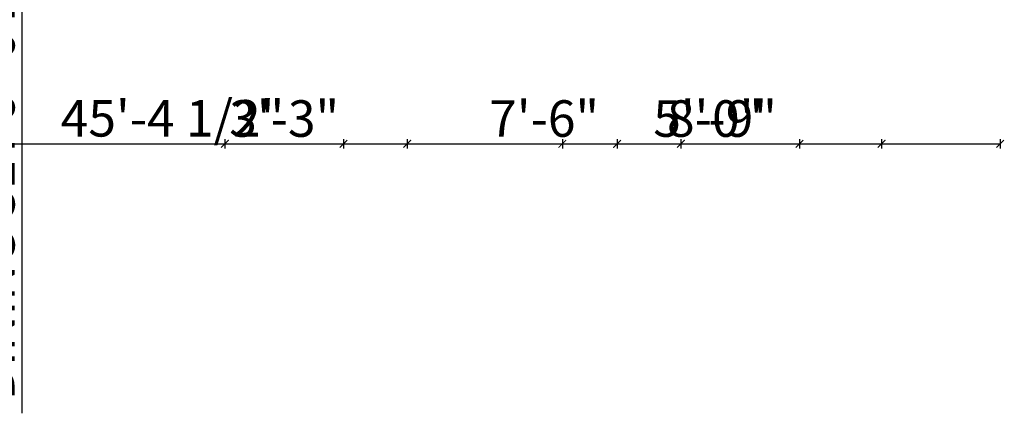
# Model space of a CAD drawing. Units: inches. Extents: x 375 to 1122, y 27 to 1069.
# Tile 6 of 155: x 667 to 990, y 27 to 157. Entities that reach past the tile are written whole.
import ezdxf

# ---------------------------------------------------------------- set-up
doc = ezdxf.new("R2010")
doc.units = ezdxf.units.IN
doc.layers.add('A-ANNO-DIMS', color=2, linetype='Continuous', lineweight=18)
doc.styles.get("Standard").update_dxf_attribs({"font": 'arial.ttf'})
doc.dimstyles.new('ISO-25', dxfattribs={"dimtxt": 12, "dimasz": 2.5, "dimexe": 1.5, "dimexo": 1.5, "dimtad": 1, "dimdec": 1, "dimlunit": 3, "dimtxsty": 'Standard', "dimblk": 'ARCHTICK', "dimcen": 2.5, "dimadec": 0, "dimazin": 0, "dimtfac": 1, "dimtdec": 1, "dimtmove": 0, "dimatfit": 3, "dimfxl": 1.5, "dimfxlon": 1, "dimarcsym": 0})

# ---------------------------------------------------------------- blocks, each defined once
blk = doc.blocks.new('_ArchTick')
at = {"color": 0, "linetype": 'ByBlock', "const_width": 0.15}
blk.add_lwpolyline([(-0.5, -0.5), (0.5, 0.5)], dxfattribs=at)
blk = doc.blocks.new('*D59')
at = {"layer": 'A-ANNO-DIMS', "color": 0, "lineweight": -2, "transparency": 16777216}
for p, q in [((668.72, 346.85), (665.72, 346.85)), ((667.22, 346.85), (667.22, 232.35)), ((668.72, 232.35), (665.72, 232.35)), ((667.22, 232.35), (667.22, 27.5))]:
    blk.add_line(p, q, dxfattribs=at)
at = {"layer": 'Defpoints', "color": 0, "transparency": 16777216}
for p in [(684.39, 346.85), (667.22, 232.35), (684.39, 232.35)]:
    blk.add_point(p, dxfattribs=at)
at = {"layer": 'A-ANNO-DIMS', "color": 0, "lineweight": -2, "transparency": 16777216, "xscale": 2.5, "yscale": 2.5, "zscale": 2.5}
for p, rotation in [((667.22, 346.85), 90), ((667.22, 232.35), 270)]:
    blk.add_blockref('_ArchTick', p, dxfattribs=dict(at, rotation=rotation))
at = {"layer": 'A-ANNO-DIMS', "color": 0, "transparency": 16777216, "insert": (660.39, 128.67), "char_height": 12, "attachment_point": 5, "rotation": 90}
blk.add_mtext('DINING SET 9\'-6 1/2" TYP.', dxfattribs=at)
blk = doc.blocks.new('*D81')
at = {"layer": 'A-ANNO-DIMS', "color": 0, "lineweight": -2, "transparency": 16777216}
for p, q in [((444.51, 117.53), (444.51, 114.53)), ((989.01, 117.53), (989.01, 114.53)), ((444.51, 116.03), (989.01, 116.03))]:
    blk.add_line(p, q, dxfattribs=at)
at = {"layer": 'Defpoints', "color": 0, "transparency": 16777216}
for p in [(444.51, 187.53), (989.01, 187.53), (989.01, 116.03)]:
    blk.add_point(p, dxfattribs=at)
at = {"layer": 'A-ANNO-DIMS', "color": 0, "lineweight": -2, "transparency": 16777216, "xscale": 2.5, "yscale": 2.5, "zscale": 2.5, "rotation": 180}
blk.add_blockref('_ArchTick', (444.51, 116.03), dxfattribs=at)
at = {"layer": 'A-ANNO-DIMS', "color": 0, "lineweight": -2, "transparency": 16777216, "xscale": 2.5, "yscale": 2.5, "zscale": 2.5}
blk.add_blockref('_ArchTick', (989.01, 116.03), dxfattribs=at)
at = {"layer": 'A-ANNO-DIMS', "color": 0, "transparency": 16777216, "insert": (716.76, 122.86), "char_height": 12, "attachment_point": 5}
blk.add_mtext('45\'-4 1/2"', dxfattribs=at)
blk = doc.blocks.new('*D84')
at = {"layer": 'A-ANNO-DIMS', "color": 0, "lineweight": -2, "transparency": 16777216}
for p, q in [((845.01, 117.53), (845.01, 114.53)), ((950.01, 117.53), (950.01, 114.53)), ((845.01, 116.03), (950.01, 116.03))]:
    blk.add_line(p, q, dxfattribs=at)
at = {"layer": 'Defpoints', "color": 0, "transparency": 16777216}
for p in [(845.01, 814.53), (950.01, 814.53), (950.01, 116.03)]:
    blk.add_point(p, dxfattribs=at)
at = {"layer": 'A-ANNO-DIMS', "color": 0, "lineweight": -2, "transparency": 16777216, "xscale": 2.5, "yscale": 2.5, "zscale": 2.5, "rotation": 180}
blk.add_blockref('_ArchTick', (845.01, 116.03), dxfattribs=at)
at = {"layer": 'A-ANNO-DIMS', "color": 0, "lineweight": -2, "transparency": 16777216, "xscale": 2.5, "yscale": 2.5, "zscale": 2.5}
blk.add_blockref('_ArchTick', (950.01, 116.03), dxfattribs=at)
at = {"layer": 'A-ANNO-DIMS', "color": 0, "transparency": 16777216, "insert": (897.51, 122.78), "char_height": 12, "attachment_point": 5}
blk.add_mtext('8\'-9"', dxfattribs=at)
blk = doc.blocks.new('*D87')
at = {"layer": 'A-ANNO-DIMS', "color": 0, "lineweight": -2, "transparency": 16777216}
for p, q in [((794.01, 117.53), (794.01, 114.53)), ((884.01, 117.53), (884.01, 114.53)), ((794.01, 116.03), (884.01, 116.03))]:
    blk.add_line(p, q, dxfattribs=at)
at = {"layer": 'Defpoints', "color": 0, "transparency": 16777216}
for p in [(794.01, 583.53), (884.01, 583.53), (884.01, 116.03)]:
    blk.add_point(p, dxfattribs=at)
at = {"layer": 'A-ANNO-DIMS', "color": 0, "lineweight": -2, "transparency": 16777216, "xscale": 2.5, "yscale": 2.5, "zscale": 2.5, "rotation": 180}
blk.add_blockref('_ArchTick', (794.01, 116.03), dxfattribs=at)
at = {"layer": 'A-ANNO-DIMS', "color": 0, "lineweight": -2, "transparency": 16777216, "xscale": 2.5, "yscale": 2.5, "zscale": 2.5}
blk.add_blockref('_ArchTick', (884.01, 116.03), dxfattribs=at)
at = {"layer": 'A-ANNO-DIMS', "color": 0, "transparency": 16777216, "insert": (839.01, 122.78), "char_height": 12, "attachment_point": 5}
blk.add_mtext('7\'-6"', dxfattribs=at)
blk = doc.blocks.new('*D89')
at = {"layer": 'A-ANNO-DIMS', "color": 0, "lineweight": -2, "transparency": 16777216}
for p, q in [((863.01, 117.53), (863.01, 114.53)), ((923.01, 117.53), (923.01, 114.53)), ((863.01, 116.03), (923.01, 116.03))]:
    blk.add_line(p, q, dxfattribs=at)
at = {"layer": 'Defpoints', "color": 0, "transparency": 16777216}
for p in [(863.01, 574.53), (923.01, 574.53), (923.01, 116.03)]:
    blk.add_point(p, dxfattribs=at)
at = {"layer": 'A-ANNO-DIMS', "color": 0, "lineweight": -2, "transparency": 16777216, "xscale": 2.5, "yscale": 2.5, "zscale": 2.5, "rotation": 180}
blk.add_blockref('_ArchTick', (863.01, 116.03), dxfattribs=at)
at = {"layer": 'A-ANNO-DIMS', "color": 0, "lineweight": -2, "transparency": 16777216, "xscale": 2.5, "yscale": 2.5, "zscale": 2.5}
blk.add_blockref('_ArchTick', (923.01, 116.03), dxfattribs=at)
at = {"layer": 'A-ANNO-DIMS', "color": 0, "transparency": 16777216, "insert": (893.01, 122.78), "char_height": 12, "attachment_point": 5}
blk.add_mtext('5\'-0"', dxfattribs=at)
blk = doc.blocks.new('*D94')
at = {"layer": 'A-ANNO-DIMS', "color": 0, "lineweight": -2, "transparency": 16777216}
for p, q in [((734.01, 117.53), (734.01, 114.53)), ((773.01, 117.53), (773.01, 114.53)), ((734.01, 116.03), (773.01, 116.03))]:
    blk.add_line(p, q, dxfattribs=at)
at = {"layer": 'Defpoints', "color": 0, "transparency": 16777216}
for p in [(734.01, 667.53), (773.01, 667.53), (773.01, 116.03)]:
    blk.add_point(p, dxfattribs=at)
at = {"layer": 'A-ANNO-DIMS', "color": 0, "lineweight": -2, "transparency": 16777216, "xscale": 2.5, "yscale": 2.5, "zscale": 2.5, "rotation": 180}
blk.add_blockref('_ArchTick', (734.01, 116.03), dxfattribs=at)
at = {"layer": 'A-ANNO-DIMS', "color": 0, "lineweight": -2, "transparency": 16777216, "xscale": 2.5, "yscale": 2.5, "zscale": 2.5}
blk.add_blockref('_ArchTick', (773.01, 116.03), dxfattribs=at)
at = {"layer": 'A-ANNO-DIMS', "color": 0, "transparency": 16777216, "insert": (753.51, 122.78), "char_height": 12, "attachment_point": 5}
blk.add_mtext('3\'-3"', dxfattribs=at)

msp = doc.modelspace()

# ---------------------------------------------------------------- dimensions: what is measured, and where the dimension line sits
at = {"layer": 'A-ANNO-DIMS'}
for base, p1, p2, picture, middle in [((950.01, 116.03), (845.01, 814.53), (950.01, 814.53), '*D84', (897.51, 122.78)), ((773.01, 116.03), (734.01, 667.53), (773.01, 667.53), '*D94', (753.51, 122.78)), ((884.01, 116.03), (794.01, 583.53), (884.01, 583.53), '*D87', (839.01, 122.78)), ((923.01, 116.03), (863.01, 574.53), (923.01, 574.53), '*D89', (893.01, 122.78)), ((989.01, 116.03), (444.51, 187.53), (989.01, 187.53), '*D81', (716.76, 122.86))]:
    dim = msp.add_linear_dim(base=base, p1=p1, p2=p2, dimstyle='ISO-25', override={"dimdec": 1, "dimlfac": 1, "dimrnd": 0, "dimzin": 1, "dimdsep": 46, "dimlunit": 4, "dimfrac": 2}, dxfattribs=at)
    dim.commit()
    dim.dimension.update_dxf_attribs({"geometry": picture, "text_midpoint": middle})
dim = msp.add_linear_dim(base=(667.22, 232.35), p1=(684.39, 346.85), p2=(684.39, 232.35), angle=270, text='DINING SET <> TYP.', dimstyle='ISO-25', override={"dimdec": 1, "dimlfac": 1, "dimrnd": 0, "dimzin": 1, "dimdsep": 46, "dimlunit": 4, "dimfrac": 2}, dxfattribs=at)
dim.commit()
dim.dimension.update_dxf_attribs({"geometry": '*D59', "text_midpoint": (660.39, 128.67)})

doc.saveas('drawing.dxf')
